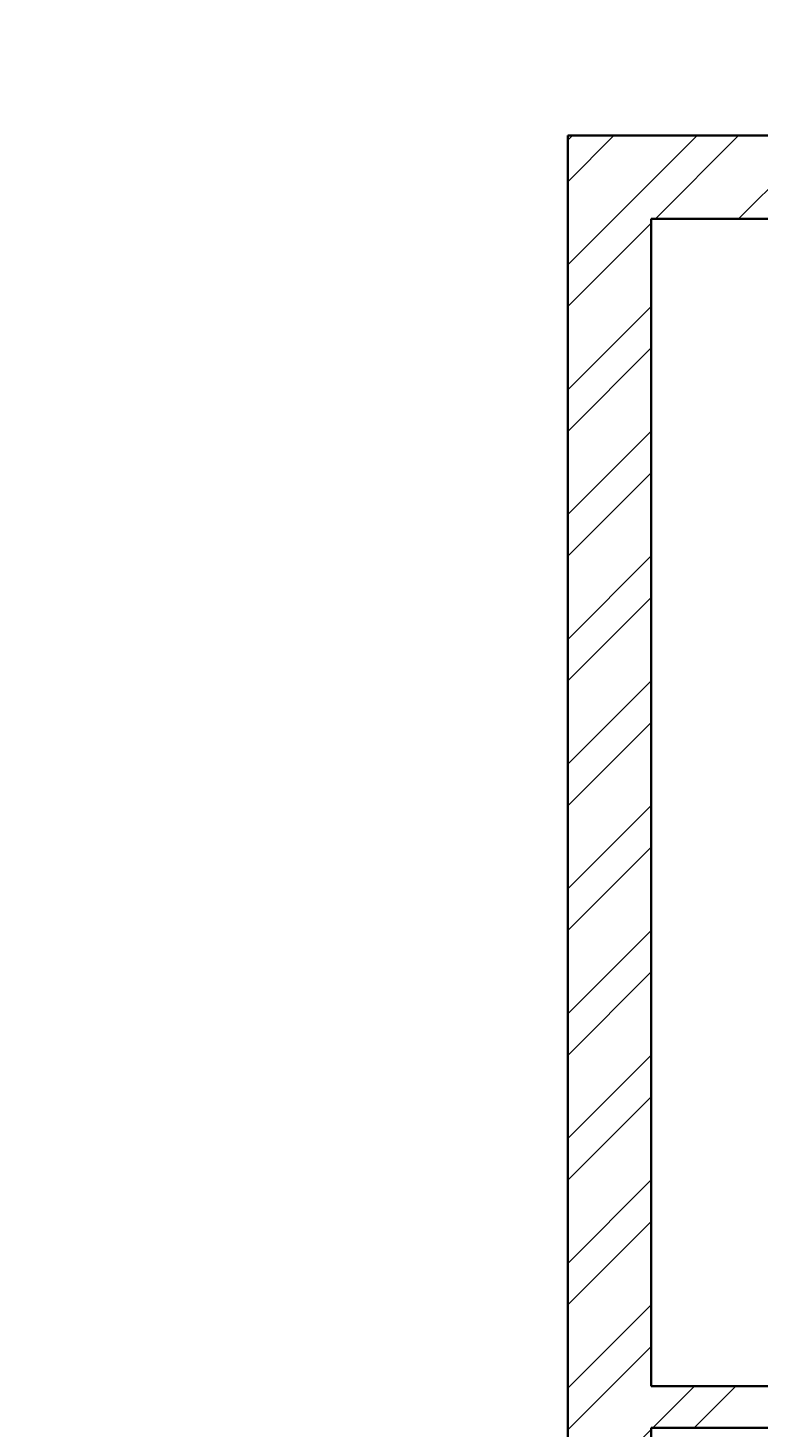
# Model space of a CAD drawing. Units: inches. Extents: x 2120 to 4013, y 1390 to 3019.
# Tile 39 of 59: x 2657 to 2736, y 2213 to 2364. Entities that reach past the tile are written whole.
import ezdxf

# ---------------------------------------------------------------- set-up
doc = ezdxf.new("R2010")
doc.units = ezdxf.units.IN
for name, color, linetype, lineweight in [('A-ANNO-DIMS', 2, 'Continuous', 18), ('A-WALL', 7, 'Continuous', 35), ('A-WALL-PATT', 252, 'Continuous', 13)]:
    doc.layers.add(name, color=color, linetype=linetype, lineweight=lineweight)
doc.styles.get("Standard").update_dxf_attribs({"font": 'arial.ttf'})
doc.dimstyles.get("Standard").update_dxf_attribs({"dimtxt": 0.18, "dimasz": 0.18, "dimexe": 0.18, "dimexo": 0.0625, "dimgap": 0.09, "dimtad": 0, "dimtih": 1, "dimtoh": 1, "dimdec": 4, "dimzin": 0, "dimdsep": 46, "dimtxsty": 'Standard', "dimcen": 0.09, "dimadec": 0, "dimazin": 0, "dimtfac": 1, "dimtdec": 4, "dimtofl": 0, "dimtmove": 0, "dimatfit": 3, "dimfxl": 1, "dimtolj": 1, "dimtzin": 0, "dimarcsym": 0})

# ---------------------------------------------------------------- blocks, each defined once
blk = doc.blocks.new('*D211')
at = {"layer": 'A-ANNO-DIMS', "color": 0, "lineweight": -2, "transparency": 16777216}
for p, q in [((2262.73, 2352.59), (2262.73, 2397.71)), ((2262.91, 2397.53), (2635.95, 2397.53)), ((3009.55, 2397.53), (2636.52, 2397.53)), ((3009.73, 2352.59), (3009.73, 2397.71))]:
    blk.add_line(p, q, dxfattribs=at)
at = {"layer": 'A-ANNO-DIMS', "color": 0, "transparency": 16777216}
for points in [[(2262.91, 2397.56), (2262.91, 2397.5), (2262.73, 2397.53)], [(3009.55, 2397.56), (3009.55, 2397.5), (3009.73, 2397.53)]]:
    blk.add_solid(points, dxfattribs=at)
at = {"layer": 'Defpoints', "color": 0, "transparency": 16777216}
for p in [(3009.73, 2397.53), (2262.73, 2352.53), (3009.73, 2352.53)]:
    blk.add_point(p, dxfattribs=at)
at = {"layer": 'A-ANNO-DIMS', "color": 0, "transparency": 16777216, "insert": (2636.23, 2397.53), "char_height": 0.18, "attachment_point": 5}
blk.add_mtext('\\A1;747', dxfattribs=at)

msp = doc.modelspace()

# ---------------------------------------------------------------- hatches: boundary and pattern name
at = {"layer": 'A-WALL-PATT'}
h = msp.add_hatch(dxfattribs=at)
h.set_pattern_fill('ANSI32', color=256)
h.paths.add_polyline_path([(2271.7331, 2343.531), (2283.3788, 2343.531), (2283.3788, 2348.031), (2283.3788, 2352.5306), (2262.7331, 2352.5306), (2262.7331, 2182.638), (2267.2331, 2182.638), (2271.7331, 2182.638), (2271.7331, 2219.031), (2391.7331, 2219.031), (2391.7331, 2214.189), (2393.9831, 2214.189), (2396.2331, 2214.189), (2396.2331, 2219.031), (2420.2331, 2219.031), (2420.2331, 2225.7535), (2417.2197, 2225.7535), (2415.7331, 2225.7535), (2415.7331, 2223.5306), (2271.7331, 2223.5306)])
h.paths.add_polyline_path([(2380.0942, 2352.5306), (2343.3788, 2352.5306), (2343.3788, 2343.531), (2363.2331, 2343.531), (2363.2331, 2288.8489), (2365.4831, 2288.8489), (2367.7331, 2288.8489), (2367.7331, 2343.531), (2380.0942, 2343.531)], flags=17)
h.paths.add_polyline_path([(2432.4339, 2352.5306), (2404.0943, 2352.5306), (2404.0943, 2343.531), (2415.7331, 2343.531), (2415.7331, 2264.0306), (2367.7331, 2264.0306), (2367.7331, 2266.4872), (2363.2331, 2266.4872), (2363.2331, 2259.531), (2367.7331, 2259.531), (2415.7331, 2259.531), (2415.7331, 2255.0658), (2420.2331, 2255.0658), (2420.2331, 2259.531), (2424.5717, 2259.531), (2424.5717, 2261.781), (2424.5717, 2264.0306), (2420.2331, 2264.0306), (2420.2331, 2343.531), (2432.4339, 2343.531)])
h.paths.add_polyline_path([(2508.9115, 2352.5306), (2456.4339, 2352.5306), (2456.4339, 2343.531), (2468.2331, 2343.531), (2468.2331, 2264.0306), (2448.0487, 2264.0306), (2448.0487, 2259.531), (2468.2331, 2259.531), (2468.2331, 2255.5496), (2472.7331, 2255.5496), (2472.7331, 2343.531), (2508.9115, 2343.531)])
h.paths.add_polyline_path([(2637.7331, 2352.5306), (2544.9116, 2352.5306), (2544.9116, 2343.531), (2589.7331, 2343.531), (2633.2331, 2343.531), (2637.7331, 2343.531)])
h.paths.add_polyline_path([(2594.2331, 2343.5306), (2589.7331, 2343.5306), (2589.7331, 2259.5306), (2589.7331, 2252.4915), (2591.9831, 2252.4915), (2594.2331, 2252.4915)])
h.paths.add_polyline_path([(2637.7331, 2223.5306), (2594.2331, 2223.5306), (2594.2331, 2230.1988), (2591.9831, 2230.1988), (2589.7331, 2230.1988), (2589.7331, 2223.5306), (2472.7331, 2223.5306), (2468.2331, 2223.5306), (2468.2331, 2219.031), (2628.7331, 2219.031), (2628.7331, 2138.031), (2637.7331, 2138.031)])
h.paths.add_polyline_path([(3822.6535, 2458.4402), (3874.9468, 2458.4402), (3874.9468, 2476.9866), (3822.6535, 2476.9866)], flags=9)
h.paths.add_polyline_path([(3834.6921, 2781.8174), (3935.9206, 2781.8174), (3935.9206, 2800.3638), (3834.6921, 2800.3638)], flags=9)
h.paths.add_polyline_path([(3832.2843, 2837.9683), (3884.5776, 2837.9683), (3884.5776, 2856.5146), (3832.2843, 2856.5146)], flags=9)
h.paths.add_polyline_path([(3830.9388, 2861.4782), (3956.8958, 2861.4782), (3956.8958, 2880.0245), (3830.9388, 2880.0245)], flags=9)
h.paths.add_polyline_path([(3870.6966, 2352.5752), (3887.9272, 2352.5752), (3887.9272, 2377.3037), (3870.6966, 2377.3037)], flags=9)
h.paths.add_polyline_path([(3289.2701, 2413.161), (3435.2223, 2413.161), (3435.2223, 2450.2538), (3289.2701, 2450.2538)], flags=9)
h.paths.add_polyline_path([(2487.6944, 2414.3601), (2637.8335, 2414.3601), (2637.8335, 2451.4528), (2487.6944, 2451.4528)], flags=9)
h.paths.add_polyline_path([(2567.3724, 1457.9199), (2815.296, 1457.9199), (2815.296, 1495.0127), (2567.3724, 1495.0127)], flags=9)
h.paths.add_polyline_path([(2655.3825, 2093.2363), (2685.9555, 2093.2363), (2685.9555, 2111.8937), (2655.3825, 2111.8937)], flags=9)
h.paths.add_polyline_path([(2543.9218, 1550.6671), (2587.8406, 1550.6671), (2587.8406, 1569.3244), (2543.9218, 1569.3244)], flags=9)
h.paths.add_polyline_path([(2905.1384, 1543.8113), (2949.0572, 1543.8113), (2949.0572, 1562.4686), (2905.1384, 1562.4686)], flags=9)
h.paths.add_polyline_path([(2736.4118, 1702.4736), (2784.2153, 1702.4736), (2784.2153, 1721.1309), (2736.4118, 1721.1309)], flags=9)
h.paths.add_polyline_path([(2912.8666, 1710.4168), (2951.707, 1710.4168), (2951.707, 1729.0741), (2912.8666, 1729.0741)], flags=9)
h.paths.add_polyline_path([(2923.5785, 1763.5038), (2959.7279, 1763.5038), (2959.7279, 1782.1611), (2923.5785, 1782.1611)], flags=9)
h.paths.add_polyline_path([(2925.2114, 1809.6137), (2967.1861, 1809.6137), (2967.1861, 1828.271), (2925.2114, 1828.271)], flags=9)
h.paths.add_polyline_path([(2996.2711, 1878.9003), (2996.2711, 1913.109), (2977.6138, 1913.109), (2977.6138, 1878.9003)], flags=9)
h.paths.add_polyline_path([(2883.0859, 1895.7192), (2927.1855, 1895.7192), (2927.1855, 1914.3766), (2883.0859, 1914.3766)], flags=9)
h.paths.add_polyline_path([(2787.3924, 1810.8013), (2841.0213, 1810.8013), (2841.0213, 1829.4587), (2787.3924, 1829.4587)], flags=9)
h.paths.add_polyline_path([(2775.6399, 2101.7395), (2829.2689, 2101.7395), (2829.2689, 2120.3968), (2775.6399, 2120.3968)], flags=9)
h.paths.add_polyline_path([(2913.0263, 2075.817), (2951.8667, 2075.817), (2951.8667, 2094.4744), (2913.0263, 2094.4744)], flags=9)
h.paths.add_polyline_path([(2929.966, 2133.3669), (2966.1154, 2133.3669), (2966.1154, 2152.0243), (2929.966, 2152.0243)], flags=9)
h.paths.add_polyline_path([(2932.7502, 2182.6088), (2968.8996, 2182.6088), (2968.8996, 2201.2662), (2932.7502, 2201.2662)], flags=9)
h.paths.add_polyline_path([(2996.0681, 2266.3173), (2996.0681, 2300.5261), (2977.4108, 2300.5261), (2977.4108, 2266.3173)], flags=9)
h.paths.add_polyline_path([(2885.1039, 2279.2186), (2929.2035, 2279.2186), (2929.2035, 2297.8759), (2885.1039, 2297.8759)], flags=9)
h.paths.add_polyline_path([(2735.7042, 2218.3197), (2783.5078, 2218.3197), (2783.5078, 2236.9771), (2735.7042, 2236.9771)], flags=9)
h.paths.add_polyline_path([(2635.6049, 2044.0085), (2648.9678, 2044.0085), (2648.9678, 2054.312), (2635.6049, 2054.312)], flags=9)
h.paths.add_polyline_path([(2714.0148, 1923.0473), (2727.3777, 1923.0473), (2727.3777, 1933.3508), (2714.0148, 1933.3508)], flags=9)
h.paths.add_polyline_path([(2709.0345, 1988.1628), (2722.3974, 1988.1628), (2722.3974, 1998.4663), (2709.0345, 1998.4663)], flags=9)
h.paths.add_polyline_path([(2592.8935, 1962.1763), (2606.2564, 1962.1763), (2606.2564, 1972.4799), (2592.8935, 1972.4799)], flags=9)
h.paths.add_polyline_path([(2618.3996, 1985.9724), (2644.1942, 1985.9724), (2644.1942, 1996.2759), (2618.3996, 1996.2759)], flags=9)
h.paths.add_polyline_path([(2601.279, 1920.5869), (2614.6419, 1920.5869), (2614.6419, 1930.8904), (2601.279, 1930.8904)], flags=9)
h.paths.add_polyline_path([(2692.3278, 1932.7645), (2704.5311, 1932.7645), (2704.5311, 1943.0681), (2692.3278, 1943.0681)], flags=9)
h.paths.add_polyline_path([(2311.122, 1672.7318), (2355.0408, 1672.7318), (2355.0408, 1691.3892), (2311.122, 1691.3892)], flags=9)
h.paths.add_polyline_path([(2456.2551, 1632.3198), (2492.4796, 1632.3198), (2492.4796, 1650.9772), (2456.2551, 1650.9772)], flags=9)
h.paths.add_polyline_path([(2401.0766, 1631.4793), (2437.301, 1631.4793), (2437.301, 1650.1367), (2401.0766, 1650.1367)], flags=9)
h.paths.add_polyline_path([(2546.7054, 1700.9235), (2594.509, 1700.9235), (2594.509, 1719.5809), (2546.7054, 1719.5809)], flags=9)
h.paths.add_polyline_path([(2445.4866, 1766.9937), (2497.5261, 1766.9937), (2497.5261, 1785.651), (2445.4866, 1785.651)], flags=9)
h.paths.add_polyline_path([(2287.9992, 1739.7675), (2326.8396, 1739.7675), (2326.8396, 1758.4248), (2287.9992, 1758.4248)], flags=9)
h.paths.add_polyline_path([(2458.5279, 1924.7607), (2510.5675, 1924.7607), (2510.5675, 1943.4181), (2458.5279, 1943.4181)], flags=9)
h.paths.add_polyline_path([(2309.2811, 1902.7642), (2345.4305, 1902.7642), (2345.4305, 1921.4215), (2309.2811, 1921.4215)], flags=9)
h.paths.add_polyline_path([(2490.7554, 2018.9392), (2530.7896, 2018.9392), (2530.7896, 2037.5965), (2490.7554, 2037.5965)], flags=9)
h.paths.add_polyline_path([(2402.143, 2024.7393), (2438.5414, 2024.7393), (2438.5414, 2043.3966), (2402.143, 2043.3966)], flags=9)
h.paths.add_polyline_path([(2287.856, 1931.7926), (2326.6964, 1931.7926), (2326.6964, 1950.4499), (2287.856, 1950.4499)], flags=9)
h.paths.add_polyline_path([(2281.7979, 2193.5771), (2320.6383, 2193.5771), (2320.6383, 2212.2344), (2281.7979, 2212.2344)], flags=25)
h.paths.add_polyline_path([(2484.0754, 2093.892), (2536.115, 2093.892), (2536.115, 2112.5494), (2484.0754, 2112.5494)], flags=9)
h.paths.add_polyline_path([(2624.7948, 2281.8639), (2624.7948, 2311.4137), (2606.1375, 2311.4137), (2606.1375, 2281.8639)], flags=9)
h.paths.add_polyline_path([(2507.5036, 2290.3639), (2541.934, 2290.3639), (2541.934, 2309.0212), (2507.5036, 2309.0212)], flags=9)
h.paths.add_polyline_path([(2423.1076, 2285.2202), (2459.332, 2285.2202), (2459.332, 2303.8776), (2423.1076, 2303.8776)], flags=9)
h.paths.add_polyline_path([(2374.5467, 2289.6272), (2410.7711, 2289.6272), (2410.7711, 2308.2846), (2374.5467, 2308.2846)], flags=25)
h.paths.add_polyline_path([(2277.4907, 2227.5651), (2316.3311, 2227.5651), (2316.3311, 2246.2224), (2277.4907, 2246.2224)], flags=25)
h.paths.add_polyline_path([(2655.3825, 2093.2367), (2685.9555, 2093.2367), (2685.9555, 2111.894), (2655.3825, 2111.894)], flags=9)
h.paths.add_polyline_path([(2543.9217, 1550.6674), (2587.8406, 1550.6674), (2587.8406, 1569.3247), (2543.9217, 1569.3247)], flags=9)
h.paths.add_polyline_path([(2905.1384, 1543.8116), (2949.0572, 1543.8116), (2949.0572, 1562.4689), (2905.1384, 1562.4689)], flags=9)
h.paths.add_polyline_path([(2736.4118, 1702.4739), (2784.2153, 1702.4739), (2784.2153, 1721.1312), (2736.4118, 1721.1312)], flags=9)
h.paths.add_polyline_path([(2912.8666, 1710.4171), (2951.707, 1710.4171), (2951.707, 1729.0744), (2912.8666, 1729.0744)], flags=9)
h.paths.add_polyline_path([(2923.5785, 1763.5041), (2959.7279, 1763.5041), (2959.7279, 1782.1614), (2923.5785, 1782.1614)], flags=9)
h.paths.add_polyline_path([(2925.2114, 1809.614), (2967.1861, 1809.614), (2967.1861, 1828.2713), (2925.2114, 1828.2713)], flags=9)
h.paths.add_polyline_path([(2996.2711, 1878.9006), (2996.2711, 1913.1094), (2977.6137, 1913.1094), (2977.6137, 1878.9006)], flags=9)
h.paths.add_polyline_path([(2883.0859, 1895.7195), (2927.1855, 1895.7195), (2927.1855, 1914.3769), (2883.0859, 1914.3769)], flags=9)
h.paths.add_polyline_path([(2787.3924, 1810.8016), (2841.0213, 1810.8016), (2841.0213, 1829.459), (2787.3924, 1829.459)], flags=9)
h.paths.add_polyline_path([(2775.6399, 2101.7398), (2829.2688, 2101.7398), (2829.2688, 2120.3971), (2775.6399, 2120.3971)], flags=9)
h.paths.add_polyline_path([(2913.0263, 2075.8173), (2951.8667, 2075.8173), (2951.8667, 2094.4747), (2913.0263, 2094.4747)], flags=9)
h.paths.add_polyline_path([(2929.966, 2133.3672), (2966.1154, 2133.3672), (2966.1154, 2152.0246), (2929.966, 2152.0246)], flags=9)
h.paths.add_polyline_path([(2932.7502, 2182.6091), (2968.8996, 2182.6091), (2968.8996, 2201.2665), (2932.7502, 2201.2665)], flags=9)
h.paths.add_polyline_path([(2996.0681, 2266.3176), (2996.0681, 2300.5264), (2977.4108, 2300.5264), (2977.4108, 2266.3176)], flags=9)
h.paths.add_polyline_path([(2885.1039, 2279.2189), (2929.2035, 2279.2189), (2929.2035, 2297.8762), (2885.1039, 2297.8762)], flags=9)
h.paths.add_polyline_path([(2735.7042, 2218.32), (2783.5078, 2218.32), (2783.5078, 2236.9774), (2735.7042, 2236.9774)], flags=9)
h.paths.add_polyline_path([(2635.6048, 2044.0088), (2648.9677, 2044.0088), (2648.9677, 2054.3123), (2635.6048, 2054.3123)], flags=9)
h.paths.add_polyline_path([(2714.0148, 1923.0476), (2727.3777, 1923.0476), (2727.3777, 1933.3511), (2714.0148, 1933.3511)], flags=9)
h.paths.add_polyline_path([(2709.0345, 1988.1631), (2722.3974, 1988.1631), (2722.3974, 1998.4666), (2709.0345, 1998.4666)], flags=9)
h.paths.add_polyline_path([(2592.8935, 1962.1766), (2606.2564, 1962.1766), (2606.2564, 1972.4802), (2592.8935, 1972.4802)], flags=9)
h.paths.add_polyline_path([(2618.3995, 1985.9727), (2644.1942, 1985.9727), (2644.1942, 1996.2762), (2618.3995, 1996.2762)], flags=9)
h.paths.add_polyline_path([(2601.279, 1920.5872), (2614.6419, 1920.5872), (2614.6419, 1930.8908), (2601.279, 1930.8908)], flags=9)
h.paths.add_polyline_path([(2692.3278, 1932.7648), (2704.5311, 1932.7648), (2704.5311, 1943.0684), (2692.3278, 1943.0684)], flags=9)
h.paths.add_polyline_path([(2311.122, 1672.7321), (2355.0408, 1672.7321), (2355.0408, 1691.3895), (2311.122, 1691.3895)], flags=9)
h.paths.add_polyline_path([(2456.2551, 1632.3201), (2492.4795, 1632.3201), (2492.4795, 1650.9775), (2456.2551, 1650.9775)], flags=9)
h.paths.add_polyline_path([(2401.0766, 1631.4796), (2437.301, 1631.4796), (2437.301, 1650.137), (2401.0766, 1650.137)], flags=9)
h.paths.add_polyline_path([(2546.7054, 1700.9238), (2594.509, 1700.9238), (2594.509, 1719.5812), (2546.7054, 1719.5812)], flags=9)
h.paths.add_polyline_path([(2445.4866, 1766.994), (2497.5261, 1766.994), (2497.5261, 1785.6513), (2445.4866, 1785.6513)], flags=9)
h.paths.add_polyline_path([(2287.9992, 1739.7678), (2326.8396, 1739.7678), (2326.8396, 1758.4251), (2287.9992, 1758.4251)], flags=9)
h.paths.add_polyline_path([(2458.5279, 1924.7611), (2510.5675, 1924.7611), (2510.5675, 1943.4184), (2458.5279, 1943.4184)], flags=9)
h.paths.add_polyline_path([(2309.2811, 1902.7645), (2345.4305, 1902.7645), (2345.4305, 1921.4218), (2309.2811, 1921.4218)], flags=9)
h.paths.add_polyline_path([(2490.7554, 2018.9395), (2530.7895, 2018.9395), (2530.7895, 2037.5968), (2490.7554, 2037.5968)], flags=9)
h.paths.add_polyline_path([(2402.143, 2024.7396), (2438.5413, 2024.7396), (2438.5413, 2043.3969), (2402.143, 2043.3969)], flags=9)
h.paths.add_polyline_path([(2287.856, 1931.7929), (2326.6964, 1931.7929), (2326.6964, 1950.4502), (2287.856, 1950.4502)], flags=9)
h.paths.add_polyline_path([(2281.7979, 2193.5774), (2320.6383, 2193.5774), (2320.6383, 2212.2347), (2281.7979, 2212.2347)], flags=25)
h.paths.add_polyline_path([(2484.0754, 2093.8924), (2536.115, 2093.8924), (2536.115, 2112.5497), (2484.0754, 2112.5497)], flags=9)
h.paths.add_polyline_path([(2624.7948, 2281.8642), (2624.7948, 2311.414), (2606.1374, 2311.414), (2606.1374, 2281.8642)], flags=9)
h.paths.add_polyline_path([(2507.5035, 2290.3642), (2541.934, 2290.3642), (2541.934, 2309.0215), (2507.5035, 2309.0215)], flags=9)
h.paths.add_polyline_path([(2423.1075, 2285.2205), (2459.332, 2285.2205), (2459.332, 2303.8779), (2423.1075, 2303.8779)], flags=9)
h.paths.add_polyline_path([(2374.5467, 2289.6275), (2410.7711, 2289.6275), (2410.7711, 2308.2849), (2374.5467, 2308.2849)], flags=25)
h.paths.add_polyline_path([(2277.4907, 2227.5654), (2316.3311, 2227.5654), (2316.3311, 2246.2227), (2277.4907, 2246.2227)], flags=25)
h = msp.add_hatch(dxfattribs=at)
h.set_pattern_fill('ANSI32', color=256)
h.paths.add_polyline_path([(2271.7331, 1980.389), (2262.7331, 1980.389), (2262.7331, 1912.8434), (2267.2331, 1912.8434), (2271.7331, 1912.8434), (2271.7331, 1922.531), (2351.2331, 1922.531), (2351.2331, 1901.4728), (2355.7331, 1901.4728), (2355.7331, 1922.531), (2357.9815, 1922.531), (2357.9815, 1926.5306), (2271.7331, 1926.5306)])
h.paths.add_polyline_path([(2589.2331, 1949.1622), (2584.7331, 1949.1622), (2580.2331, 1949.1622), (2580.2331, 1874.5306), (2355.7331, 1874.5306), (2355.7331, 1880.1922), (2351.2331, 1880.1922), (2351.2331, 1874.5306), (2271.7331, 1874.5306), (2271.7331, 1888.8431), (2262.7331, 1888.8431), (2262.7331, 1842.2909), (2267.2331, 1842.2909), (2271.7331, 1842.2909), (2271.7331, 1865.531), (2415.7331, 1865.531), (2415.7331, 1779.7286), (2420.2331, 1779.7286), (2420.2331, 1865.531), (2589.2331, 1865.531)])
h.paths.add_polyline_path([(2271.7331, 1782.2906), (2262.7331, 1782.2906), (2262.7331, 1711.4639), (2267.2331, 1711.4639), (2271.7331, 1711.4639), (2271.7331, 1738.031), (2420.2331, 1738.031), (2420.2331, 1742.531), (2420.2331, 1747.3376), (2417.9831, 1747.3376), (2415.7331, 1747.3376), (2415.7331, 1742.5306), (2271.7331, 1742.5306)])
h.paths.add_polyline_path([(2271.7331, 1627.031), (2362.3957, 1627.031), (2362.3957, 1629.281), (2362.3957, 1631.5306), (2271.7331, 1631.5306), (2271.7331, 1675.4636), (2262.7331, 1675.4636), (2262.7331, 1581.531), (2405.3032, 1581.531), (2405.3032, 1586.031), (2405.3032, 1590.5306), (2396.2331, 1590.5306), (2396.2331, 1691.4513), (2418.7206, 1691.4513), (2418.7206, 1695.951), (2396.2331, 1695.951), (2391.7331, 1695.951), (2391.7331, 1631.5306), (2386.7425, 1631.5306), (2386.7425, 1629.2806), (2386.7425, 1627.031), (2391.7331, 1627.031), (2391.7331, 1586.1709), (2271.7331, 1586.1709)])
h.paths.add_polyline_path([(2459.6703, 1590.5306), (2429.3032, 1590.5306), (2429.3032, 1581.531), (2459.6703, 1581.531), (2459.6703, 1586.031)])
h.paths.add_polyline_path([(2501.2331, 1590.531), (2501.2331, 1665.0195), (2498.9831, 1665.0195), (2496.7331, 1665.0195), (2496.7331, 1590.5306), (2483.8201, 1590.5306), (2483.8201, 1590.1579), (2483.6704, 1590.1579), (2483.6704, 1581.531), (2505.0196, 1581.531), (2505.0196, 1583.781), (2505.0196, 1586.0306), (2501.2331, 1586.0306)])
h.paths.add_polyline_path([(2544.1361, 1583.781), (2544.1361, 1586.0306), (2527.1368, 1586.0306), (2527.1368, 1583.7806), (2527.1368, 1581.531), (2544.1361, 1581.531)])
h.paths.add_polyline_path([(3822.6535, 2458.4402), (3874.9468, 2458.4402), (3874.9468, 2476.9866), (3822.6535, 2476.9866)], flags=9)
h.paths.add_polyline_path([(3834.6921, 2781.8174), (3935.9206, 2781.8174), (3935.9206, 2800.3638), (3834.6921, 2800.3638)], flags=9)
h.paths.add_polyline_path([(3832.2843, 2837.9683), (3884.5776, 2837.9683), (3884.5776, 2856.5146), (3832.2843, 2856.5146)], flags=9)
h.paths.add_polyline_path([(3830.9388, 2861.4782), (3956.8958, 2861.4782), (3956.8958, 2880.0245), (3830.9388, 2880.0245)], flags=9)
h.paths.add_polyline_path([(3870.6966, 2352.5752), (3887.9272, 2352.5752), (3887.9272, 2377.3037), (3870.6966, 2377.3037)], flags=9)
h.paths.add_polyline_path([(3289.2701, 2413.161), (3435.2223, 2413.161), (3435.2223, 2450.2538), (3289.2701, 2450.2538)], flags=9)
h.paths.add_polyline_path([(2487.6944, 2414.3601), (2637.8335, 2414.3601), (2637.8335, 2451.4528), (2487.6944, 2451.4528)], flags=9)
h.paths.add_polyline_path([(2567.3724, 1457.9199), (2815.296, 1457.9199), (2815.296, 1495.0127), (2567.3724, 1495.0127)], flags=9)
h.paths.add_polyline_path([(2655.3825, 2093.2363), (2685.9555, 2093.2363), (2685.9555, 2111.8937), (2655.3825, 2111.8937)], flags=9)
h.paths.add_polyline_path([(2543.9218, 1550.6671), (2587.8406, 1550.6671), (2587.8406, 1569.3244), (2543.9218, 1569.3244)], flags=9)
h.paths.add_polyline_path([(2905.1384, 1543.8113), (2949.0572, 1543.8113), (2949.0572, 1562.4686), (2905.1384, 1562.4686)], flags=9)
h.paths.add_polyline_path([(2736.4118, 1702.4736), (2784.2153, 1702.4736), (2784.2153, 1721.1309), (2736.4118, 1721.1309)], flags=9)
h.paths.add_polyline_path([(2912.8666, 1710.4168), (2951.707, 1710.4168), (2951.707, 1729.0741), (2912.8666, 1729.0741)], flags=9)
h.paths.add_polyline_path([(2923.5785, 1763.5038), (2959.7279, 1763.5038), (2959.7279, 1782.1611), (2923.5785, 1782.1611)], flags=9)
h.paths.add_polyline_path([(2925.2114, 1809.6137), (2967.1861, 1809.6137), (2967.1861, 1828.271), (2925.2114, 1828.271)], flags=9)
h.paths.add_polyline_path([(2996.2711, 1878.9003), (2996.2711, 1913.109), (2977.6138, 1913.109), (2977.6138, 1878.9003)], flags=9)
h.paths.add_polyline_path([(2883.0859, 1895.7192), (2927.1855, 1895.7192), (2927.1855, 1914.3766), (2883.0859, 1914.3766)], flags=9)
h.paths.add_polyline_path([(2787.3924, 1810.8013), (2841.0213, 1810.8013), (2841.0213, 1829.4587), (2787.3924, 1829.4587)], flags=9)
h.paths.add_polyline_path([(2775.6399, 2101.7395), (2829.2689, 2101.7395), (2829.2689, 2120.3968), (2775.6399, 2120.3968)], flags=9)
h.paths.add_polyline_path([(2913.0263, 2075.817), (2951.8667, 2075.817), (2951.8667, 2094.4744), (2913.0263, 2094.4744)], flags=9)
h.paths.add_polyline_path([(2929.966, 2133.3669), (2966.1154, 2133.3669), (2966.1154, 2152.0243), (2929.966, 2152.0243)], flags=9)
h.paths.add_polyline_path([(2932.7502, 2182.6088), (2968.8996, 2182.6088), (2968.8996, 2201.2662), (2932.7502, 2201.2662)], flags=9)
h.paths.add_polyline_path([(2996.0681, 2266.3173), (2996.0681, 2300.5261), (2977.4108, 2300.5261), (2977.4108, 2266.3173)], flags=9)
h.paths.add_polyline_path([(2885.1039, 2279.2186), (2929.2035, 2279.2186), (2929.2035, 2297.8759), (2885.1039, 2297.8759)], flags=9)
h.paths.add_polyline_path([(2735.7042, 2218.3197), (2783.5078, 2218.3197), (2783.5078, 2236.9771), (2735.7042, 2236.9771)], flags=9)
h.paths.add_polyline_path([(2635.6049, 2044.0085), (2648.9678, 2044.0085), (2648.9678, 2054.312), (2635.6049, 2054.312)], flags=9)
h.paths.add_polyline_path([(2714.0148, 1923.0473), (2727.3777, 1923.0473), (2727.3777, 1933.3508), (2714.0148, 1933.3508)], flags=9)
h.paths.add_polyline_path([(2709.0345, 1988.1628), (2722.3974, 1988.1628), (2722.3974, 1998.4663), (2709.0345, 1998.4663)], flags=9)
h.paths.add_polyline_path([(2592.8935, 1962.1763), (2606.2564, 1962.1763), (2606.2564, 1972.4799), (2592.8935, 1972.4799)], flags=9)
h.paths.add_polyline_path([(2618.3996, 1985.9724), (2644.1942, 1985.9724), (2644.1942, 1996.2759), (2618.3996, 1996.2759)], flags=9)
h.paths.add_polyline_path([(2601.279, 1920.5869), (2614.6419, 1920.5869), (2614.6419, 1930.8904), (2601.279, 1930.8904)], flags=9)
h.paths.add_polyline_path([(2692.3278, 1932.7645), (2704.5311, 1932.7645), (2704.5311, 1943.0681), (2692.3278, 1943.0681)], flags=9)
h.paths.add_polyline_path([(2311.122, 1672.7318), (2355.0408, 1672.7318), (2355.0408, 1691.3892), (2311.122, 1691.3892)], flags=25)
h.paths.add_polyline_path([(2456.2551, 1632.3198), (2492.4796, 1632.3198), (2492.4796, 1650.9772), (2456.2551, 1650.9772)], flags=9)
h.paths.add_polyline_path([(2401.0766, 1631.4793), (2437.301, 1631.4793), (2437.301, 1650.1367), (2401.0766, 1650.1367)], flags=9)
h.paths.add_polyline_path([(2546.7054, 1700.9235), (2594.509, 1700.9235), (2594.509, 1719.5809), (2546.7054, 1719.5809)], flags=9)
h.paths.add_polyline_path([(2445.4866, 1766.9937), (2497.5261, 1766.9937), (2497.5261, 1785.651), (2445.4866, 1785.651)], flags=9)
h.paths.add_polyline_path([(2287.9992, 1739.7675), (2326.8396, 1739.7675), (2326.8396, 1758.4248), (2287.9992, 1758.4248)], flags=24)
h.paths.add_polyline_path([(2458.5279, 1924.7607), (2510.5675, 1924.7607), (2510.5675, 1943.4181), (2458.5279, 1943.4181)], flags=25)
h.paths.add_polyline_path([(2309.2811, 1902.7642), (2345.4305, 1902.7642), (2345.4305, 1921.4215), (2309.2811, 1921.4215)], flags=25)
h.paths.add_polyline_path([(2490.7554, 2018.9392), (2530.7896, 2018.9392), (2530.7896, 2037.5965), (2490.7554, 2037.5965)], flags=9)
h.paths.add_polyline_path([(2402.143, 2024.7393), (2438.5414, 2024.7393), (2438.5414, 2043.3966), (2402.143, 2043.3966)], flags=9)
h.paths.add_polyline_path([(2287.856, 1931.7926), (2326.6964, 1931.7926), (2326.6964, 1950.4499), (2287.856, 1950.4499)], flags=25)
h.paths.add_polyline_path([(2281.7979, 2193.5771), (2320.6383, 2193.5771), (2320.6383, 2212.2344), (2281.7979, 2212.2344)], flags=9)
h.paths.add_polyline_path([(2484.0754, 2093.892), (2536.115, 2093.892), (2536.115, 2112.5494), (2484.0754, 2112.5494)], flags=9)
h.paths.add_polyline_path([(2624.7948, 2281.8639), (2624.7948, 2311.4137), (2606.1375, 2311.4137), (2606.1375, 2281.8639)], flags=9)
h.paths.add_polyline_path([(2507.5036, 2290.3639), (2541.934, 2290.3639), (2541.934, 2309.0212), (2507.5036, 2309.0212)], flags=9)
h.paths.add_polyline_path([(2423.1076, 2285.2202), (2459.332, 2285.2202), (2459.332, 2303.8776), (2423.1076, 2303.8776)], flags=9)
h.paths.add_polyline_path([(2374.5467, 2289.6272), (2410.7711, 2289.6272), (2410.7711, 2308.2846), (2374.5467, 2308.2846)], flags=9)
h.paths.add_polyline_path([(2277.4907, 2227.5651), (2316.3311, 2227.5651), (2316.3311, 2246.2224), (2277.4907, 2246.2224)], flags=9)
h.paths.add_polyline_path([(2655.3825, 2093.2367), (2685.9555, 2093.2367), (2685.9555, 2111.894), (2655.3825, 2111.894)], flags=9)
h.paths.add_polyline_path([(2543.9217, 1550.6674), (2587.8406, 1550.6674), (2587.8406, 1569.3247), (2543.9217, 1569.3247)], flags=9)
h.paths.add_polyline_path([(2905.1384, 1543.8116), (2949.0572, 1543.8116), (2949.0572, 1562.4689), (2905.1384, 1562.4689)], flags=9)
h.paths.add_polyline_path([(2736.4118, 1702.4739), (2784.2153, 1702.4739), (2784.2153, 1721.1312), (2736.4118, 1721.1312)], flags=9)
h.paths.add_polyline_path([(2912.8666, 1710.4171), (2951.707, 1710.4171), (2951.707, 1729.0744), (2912.8666, 1729.0744)], flags=9)
h.paths.add_polyline_path([(2923.5785, 1763.5041), (2959.7279, 1763.5041), (2959.7279, 1782.1614), (2923.5785, 1782.1614)], flags=9)
h.paths.add_polyline_path([(2925.2114, 1809.614), (2967.1861, 1809.614), (2967.1861, 1828.2713), (2925.2114, 1828.2713)], flags=9)
h.paths.add_polyline_path([(2996.2711, 1878.9006), (2996.2711, 1913.1094), (2977.6137, 1913.1094), (2977.6137, 1878.9006)], flags=9)
h.paths.add_polyline_path([(2883.0859, 1895.7195), (2927.1855, 1895.7195), (2927.1855, 1914.3769), (2883.0859, 1914.3769)], flags=9)
h.paths.add_polyline_path([(2787.3924, 1810.8016), (2841.0213, 1810.8016), (2841.0213, 1829.459), (2787.3924, 1829.459)], flags=9)
h.paths.add_polyline_path([(2775.6399, 2101.7398), (2829.2688, 2101.7398), (2829.2688, 2120.3971), (2775.6399, 2120.3971)], flags=9)
h.paths.add_polyline_path([(2913.0263, 2075.8173), (2951.8667, 2075.8173), (2951.8667, 2094.4747), (2913.0263, 2094.4747)], flags=9)
h.paths.add_polyline_path([(2929.966, 2133.3672), (2966.1154, 2133.3672), (2966.1154, 2152.0246), (2929.966, 2152.0246)], flags=9)
h.paths.add_polyline_path([(2932.7502, 2182.6091), (2968.8996, 2182.6091), (2968.8996, 2201.2665), (2932.7502, 2201.2665)], flags=9)
h.paths.add_polyline_path([(2996.0681, 2266.3176), (2996.0681, 2300.5264), (2977.4108, 2300.5264), (2977.4108, 2266.3176)], flags=9)
h.paths.add_polyline_path([(2885.1039, 2279.2189), (2929.2035, 2279.2189), (2929.2035, 2297.8762), (2885.1039, 2297.8762)], flags=9)
h.paths.add_polyline_path([(2735.7042, 2218.32), (2783.5078, 2218.32), (2783.5078, 2236.9774), (2735.7042, 2236.9774)], flags=9)
h.paths.add_polyline_path([(2635.6048, 2044.0088), (2648.9677, 2044.0088), (2648.9677, 2054.3123), (2635.6048, 2054.3123)], flags=9)
h.paths.add_polyline_path([(2714.0148, 1923.0476), (2727.3777, 1923.0476), (2727.3777, 1933.3511), (2714.0148, 1933.3511)], flags=9)
h.paths.add_polyline_path([(2709.0345, 1988.1631), (2722.3974, 1988.1631), (2722.3974, 1998.4666), (2709.0345, 1998.4666)], flags=9)
h.paths.add_polyline_path([(2592.8935, 1962.1766), (2606.2564, 1962.1766), (2606.2564, 1972.4802), (2592.8935, 1972.4802)], flags=9)
h.paths.add_polyline_path([(2618.3995, 1985.9727), (2644.1942, 1985.9727), (2644.1942, 1996.2762), (2618.3995, 1996.2762)], flags=9)
h.paths.add_polyline_path([(2601.279, 1920.5872), (2614.6419, 1920.5872), (2614.6419, 1930.8908), (2601.279, 1930.8908)], flags=9)
h.paths.add_polyline_path([(2692.3278, 1932.7648), (2704.5311, 1932.7648), (2704.5311, 1943.0684), (2692.3278, 1943.0684)], flags=9)
h.paths.add_polyline_path([(2311.122, 1672.7321), (2355.0408, 1672.7321), (2355.0408, 1691.3895), (2311.122, 1691.3895)], flags=25)
h.paths.add_polyline_path([(2456.2551, 1632.3201), (2492.4795, 1632.3201), (2492.4795, 1650.9775), (2456.2551, 1650.9775)], flags=9)
h.paths.add_polyline_path([(2401.0766, 1631.4796), (2437.301, 1631.4796), (2437.301, 1650.137), (2401.0766, 1650.137)], flags=9)
h.paths.add_polyline_path([(2546.7054, 1700.9238), (2594.509, 1700.9238), (2594.509, 1719.5812), (2546.7054, 1719.5812)], flags=9)
h.paths.add_polyline_path([(2445.4866, 1766.994), (2497.5261, 1766.994), (2497.5261, 1785.6513), (2445.4866, 1785.6513)], flags=9)
h.paths.add_polyline_path([(2287.9992, 1739.7678), (2326.8396, 1739.7678), (2326.8396, 1758.4251), (2287.9992, 1758.4251)], flags=24)
h.paths.add_polyline_path([(2458.5279, 1924.7611), (2510.5675, 1924.7611), (2510.5675, 1943.4184), (2458.5279, 1943.4184)], flags=25)
h.paths.add_polyline_path([(2309.2811, 1902.7645), (2345.4305, 1902.7645), (2345.4305, 1921.4218), (2309.2811, 1921.4218)], flags=25)
h.paths.add_polyline_path([(2490.7554, 2018.9395), (2530.7895, 2018.9395), (2530.7895, 2037.5968), (2490.7554, 2037.5968)], flags=9)
h.paths.add_polyline_path([(2402.143, 2024.7396), (2438.5413, 2024.7396), (2438.5413, 2043.3969), (2402.143, 2043.3969)], flags=9)
h.paths.add_polyline_path([(2287.856, 1931.7929), (2326.6964, 1931.7929), (2326.6964, 1950.4502), (2287.856, 1950.4502)], flags=25)
h.paths.add_polyline_path([(2281.7979, 2193.5774), (2320.6383, 2193.5774), (2320.6383, 2212.2347), (2281.7979, 2212.2347)], flags=9)
h.paths.add_polyline_path([(2484.0754, 2093.8924), (2536.115, 2093.8924), (2536.115, 2112.5497), (2484.0754, 2112.5497)], flags=9)
h.paths.add_polyline_path([(2624.7948, 2281.8642), (2624.7948, 2311.414), (2606.1374, 2311.414), (2606.1374, 2281.8642)], flags=9)
h.paths.add_polyline_path([(2507.5035, 2290.3642), (2541.934, 2290.3642), (2541.934, 2309.0215), (2507.5035, 2309.0215)], flags=9)
h.paths.add_polyline_path([(2423.1075, 2285.2205), (2459.332, 2285.2205), (2459.332, 2303.8779), (2423.1075, 2303.8779)], flags=9)
h.paths.add_polyline_path([(2374.5467, 2289.6275), (2410.7711, 2289.6275), (2410.7711, 2308.2849), (2374.5467, 2308.2849)], flags=9)
h.paths.add_polyline_path([(2277.4907, 2227.5654), (2316.3311, 2227.5654), (2316.3311, 2246.2227), (2277.4907, 2246.2227)], flags=9)
h = msp.add_hatch(dxfattribs=at)
h.set_pattern_fill('ANSI32', color=256)
h.paths.add_polyline_path([(2271.7331, 2122.6377), (2262.7331, 2122.6377), (2262.7331, 2040.3893), (2267.2331, 2040.3893), (2271.7331, 2040.3893), (2271.7331, 2044.8856), (2271.7331, 2070.531), (2391.7331, 2070.531), (2391.7331, 1926.5306), (2388.3993, 1926.5306), (2388.3993, 1922.531), (2395.7331, 1922.531), (2395.7331, 1992.531), (2400.4511, 1992.531), (2400.4511, 1997.0306), (2395.7331, 1997.0306), (2395.7331, 2070.531), (2443.7331, 2070.531), (2443.7331, 2046.1368), (2448.2331, 2046.1368), (2448.2331, 2070.531), (2580.2331, 2070.531), (2580.2331, 1997.0306), (2492.9076, 1997.0306), (2492.9076, 1992.531), (2580.2331, 1992.531), (2580.2331, 1983.9368), (2589.2331, 1983.9368), (2589.2331, 2070.531), (2589.2331, 2075.0306), (2396.2331, 2075.0306), (2396.2331, 2184.3565), (2393.9831, 2184.3565), (2391.7331, 2184.3565), (2391.7331, 2075.0306), (2271.7331, 2075.0306)])
h.paths.add_polyline_path([(2724.7331, 2138.0306), (2628.7331, 2138.0306), (2628.7331, 2070.5306), (2628.7331, 2067.0987), (2633.2331, 2067.0987), (2637.7331, 2067.0987), (2637.7331, 2070.531), (2657.3413, 2070.531), (2657.3413, 2079.5306), (2637.7331, 2079.5306), (2637.7331, 2129.031), (2715.7331, 2129.031), (2715.7331, 2079.5306), (2698.0378, 2079.5306), (2698.0378, 2070.531), (2715.7331, 2070.531), (2715.7331, 2012.1531), (2720.2331, 2012.1531), (2724.7331, 2012.1531)])
h.paths.add_polyline_path([(2724.7331, 2213.031), (2831.3209, 2213.031), (2831.3209, 2215.281), (2831.3209, 2217.5306), (2724.7331, 2217.5306), (2724.7331, 2343.531), (2751.8755, 2343.531), (2751.8755, 2352.5306), (2715.7331, 2352.5306), (2715.7331, 2138.031), (2724.7331, 2138.031)])
h.paths.add_polyline_path([(2902.53, 2352.5306), (2811.8755, 2352.5306), (2811.8755, 2343.531), (2867.2331, 2343.531), (2867.2331, 2217.5306), (2863.6364, 2217.5306), (2863.6364, 2213.031), (2871.7331, 2213.031), (2871.7331, 2217.531), (2871.7331, 2343.531), (2902.53, 2343.531)])
h.paths.add_polyline_path([(3009.7331, 2352.5306), (2938.53, 2352.5306), (2938.53, 2343.531), (2966.2331, 2343.531), (2966.2331, 2242.3281), (2968.4831, 2242.3281), (2970.7331, 2242.3281), (2970.7331, 2343.531), (3009.7331, 2343.531)])
h.paths.add_polyline_path([(3009.7331, 2217.5306), (2970.7331, 2217.5306), (2970.7331, 2220.5422), (2968.4831, 2220.5422), (2966.2331, 2220.5422), (2966.2331, 2217.5306), (2911.7752, 2217.5306), (2907.7331, 2217.5306), (2907.7331, 2213.0306), (2907.7331, 2194.9663), (2912.2331, 2194.9663), (2912.2331, 2213.031), (2970.7331, 2213.031), (3000.7331, 2213.031), (3000.7331, 2205.523), (3009.7331, 2205.523)])
h.paths.add_polyline_path([(3009.7331, 2181.5227), (3000.7331, 2181.5227), (3000.7331, 2165.0306), (2912.2331, 2165.0306), (2912.2331, 2170.8202), (2907.7331, 2170.8202), (2907.7331, 2165.0306), (2899.5169, 2165.0306), (2899.5169, 2162.7806), (2899.5169, 2160.531), (2907.7331, 2160.531), (2907.7331, 2137.3432), (2912.2331, 2137.3432), (2912.2331, 2160.531), (3000.7331, 2160.531), (3000.7331, 2150.4993), (3009.7331, 2150.4993)])
h.paths.add_polyline_path([(3009.7331, 2126.499), (3005.2331, 2126.499), (3000.7331, 2126.499), (3000.7331, 2112.5306), (2912.2331, 2112.5306), (2912.2331, 2115.6036), (2907.7331, 2115.6036), (2907.7331, 2108.031), (3000.7331, 2108.031), (3000.7331, 2084.7256), (3009.7331, 2084.7256)], flags=17)
h.paths.add_polyline_path([(3009.7331, 1971.531), (3009.7331, 2024.7253), (3000.7331, 2024.7253), (3000.7331, 2006.4153), (3000.7331, 1971.5306), (2864.2331, 1971.5306), (2864.2331, 2160.531), (2868.0522, 2160.531), (2868.0522, 2165.0306), (2859.7331, 2165.0306), (2859.7331, 1971.5306), (2724.7331, 1971.5306), (2724.7331, 1977.7012), (2715.7331, 1977.7012), (2715.7331, 1962.5306), (2715.7331, 1950.9035), (2720.2331, 1950.9035), (2724.7331, 1950.9035), (2724.7331, 1962.531), (2855.2331, 1962.531), (2859.7331, 1962.531), (2859.7331, 1835.031), (2864.2331, 1834.8158), (2864.2331, 1962.531), (2958.7331, 1962.531), (2958.7331, 1937.0925), (2963.2331, 1937.0925), (2963.2331, 1962.531), (3000.7331, 1962.531), (3009.7331, 1962.531)])
h.paths.add_polyline_path([(2724.7331, 1728.531), (2822.7164, 1728.531), (2822.7164, 1733.0306), (2724.7331, 1733.0306), (2724.7331, 1779.3416), (2715.7331, 1779.3416), (2715.7331, 1581.531), (2753.02, 1581.531), (2753.02, 1586.031), (2753.02, 1590.5306), (2724.7331, 1590.5306)])
h.paths.add_polyline_path([(2864.2331, 1590.531), (2864.2331, 1787.031), (2868.4075, 1787.031), (2868.4075, 1791.5306), (2859.7331, 1791.5306), (2859.7331, 1739.0306), (2859.7331, 1733.0306), (2854.3125, 1733.0306), (2854.3125, 1728.531), (2859.7331, 1728.531), (2859.7331, 1590.5306), (2813.02, 1590.5306), (2813.02, 1581.531), (2868.4123, 1581.531), (2868.4123, 1583.781), (2868.4123, 1586.0306), (2864.2331, 1586.0306)])
h.paths.add_polyline_path([(3009.7331, 1754.6619), (3000.7331, 1754.6619), (3000.7331, 1739.0306), (2912.2331, 1739.0306), (2912.2331, 1742.2257), (2907.7331, 1742.2257), (2907.7331, 1739.0306), (2907.7331, 1734.531), (3000.7331, 1734.531), (3000.7331, 1590.5306), (3000.7331, 1586.0306), (2971.3921, 1586.0306), (2971.3921, 1581.531), (3009.7331, 1581.531)])
h.paths.add_polyline_path([(2911.3921, 1583.781), (2911.3921, 1586.0306), (2891.2138, 1586.0306), (2891.2138, 1581.531), (2911.3921, 1581.531)])
h.paths.add_polyline_path([(3009.7331, 1799.8422), (3000.7331, 1799.8422), (3000.7331, 1791.5306), (2912.2331, 1791.5306), (2912.2331, 1796.3264), (2909.9831, 1796.3264), (2907.7331, 1796.3264), (2907.7331, 1791.5306), (2902.7033, 1791.5306), (2902.7033, 1787.031), (2907.7331, 1787.031), (2907.7331, 1761.1622), (2912.2331, 1761.1622), (2912.2331, 1787.031), (3000.7331, 1787.031), (3000.7331, 1778.6622), (3009.7331, 1778.6622)])
h.paths.add_polyline_path([(3009.7331, 1839.5306), (2963.2331, 1839.5306), (2963.2331, 1842.8629), (2960.9831, 1842.8629), (2958.7331, 1842.8629), (2958.7331, 1839.5306), (2907.7331, 1839.5306), (2907.7331, 1814.4599), (2912.2331, 1814.4599), (2912.2331, 1835.031), (3000.7331, 1835.031), (3000.7331, 1823.8425), (3009.7331, 1823.8425), (3009.7331, 1835.031)])
h.paths.add_polyline_path([(2963.2331, 1901.0922), (2960.9831, 1901.0922), (2958.7331, 1901.0922), (2958.7331, 1862.8843), (2963.2331, 1862.8843)], flags=17)
h.paths.add_polyline_path([(2724.7331, 1891.9826), (2724.7331, 1914.3416), (2715.7331, 1914.3416), (2715.7331, 1783.8416), (2637.7331, 1783.8416), (2637.7331, 1914.3416), (2628.7331, 1914.3416), (2624.7701, 1914.3416), (2624.7701, 1909.8416), (2624.7701, 1905.3419), (2628.7331, 1905.3419), (2628.7331, 1876.9915), (2628.7331, 1779.3419), (2637.7331, 1779.3419), (2715.7331, 1779.3419), (2724.7331, 1779.3419), (2724.7331, 1835.031)])
h.paths.add_polyline_path([(2637.7331, 1731.531), (2637.7331, 1779.3416), (2628.7331, 1779.3416), (2628.7331, 1731.5306), (2589.2331, 1731.5306), (2535.9814, 1731.5306), (2496.7331, 1731.5306), (2496.7331, 1725.6876), (2498.9831, 1725.6876), (2501.2331, 1725.6876), (2501.2331, 1727.031), (2628.7331, 1727.031), (2628.7331, 1680.4203), (2628.7331, 1590.5306), (2628.7331, 1586.0306), (2604.1361, 1586.0306), (2604.1361, 1581.531), (2637.7331, 1581.531), (2637.7331, 1590.531)])

# ---------------------------------------------------------------- linework, layer by layer
at = {"layer": 'A-WALL'}
for p, q in [((2715.7331, 2352.531), (2715.7331, 2138.031)), ((2715.7331, 2352.531), (3009.7331, 2352.531)), ((2715.7331, 2352.5306), (3009.7331, 2352.5306)), ((2715.7331, 2352.5306), (2715.7331, 2138.0306)), ((2724.7331, 2343.531), (2724.7331, 2217.531)), ((2724.7331, 2217.531), (2724.7331, 2343.531)), ((2724.7331, 2343.531), (2867.2331, 2343.531)), ((2724.7331, 2343.5306), (2867.2331, 2343.5306)), ((2724.7331, 2217.5306), (2724.7331, 2343.5306)), ((2724.7331, 2343.5306), (2724.7331, 2217.5306)), ((2724.7331, 2217.531), (2832.8684, 2217.531)), ((2724.7331, 2217.5306), (2832.8684, 2217.5306)), ((2724.7331, 2138.031), (2724.7331, 2213.031)), ((2831.3209, 2213.031), (2724.7331, 2213.031)), ((2724.7331, 2213.031), (2724.7331, 2010.5745))]:
    msp.add_line(p, q, dxfattribs=at)

# ---------------------------------------------------------------- dimensions: what is measured, and where the dimension line sits
at = {"layer": 'A-ANNO-DIMS'}
dim = msp.add_linear_dim(base=(3009.7331, 2397.531), p1=(2262.7331, 2352.531), p2=(3009.7331, 2352.531), dimstyle='Standard', override={"dimdec": 0, "dimlfac": 1, "dimrnd": 0, "dimzin": 0, "dimdsep": 46, "dimlunit": 2}, dxfattribs=at)
dim.commit()
dim.dimension.update_dxf_attribs({"geometry": '*D211', "text_midpoint": (2636.2331, 2397.531)})

doc.saveas('drawing.dxf')
